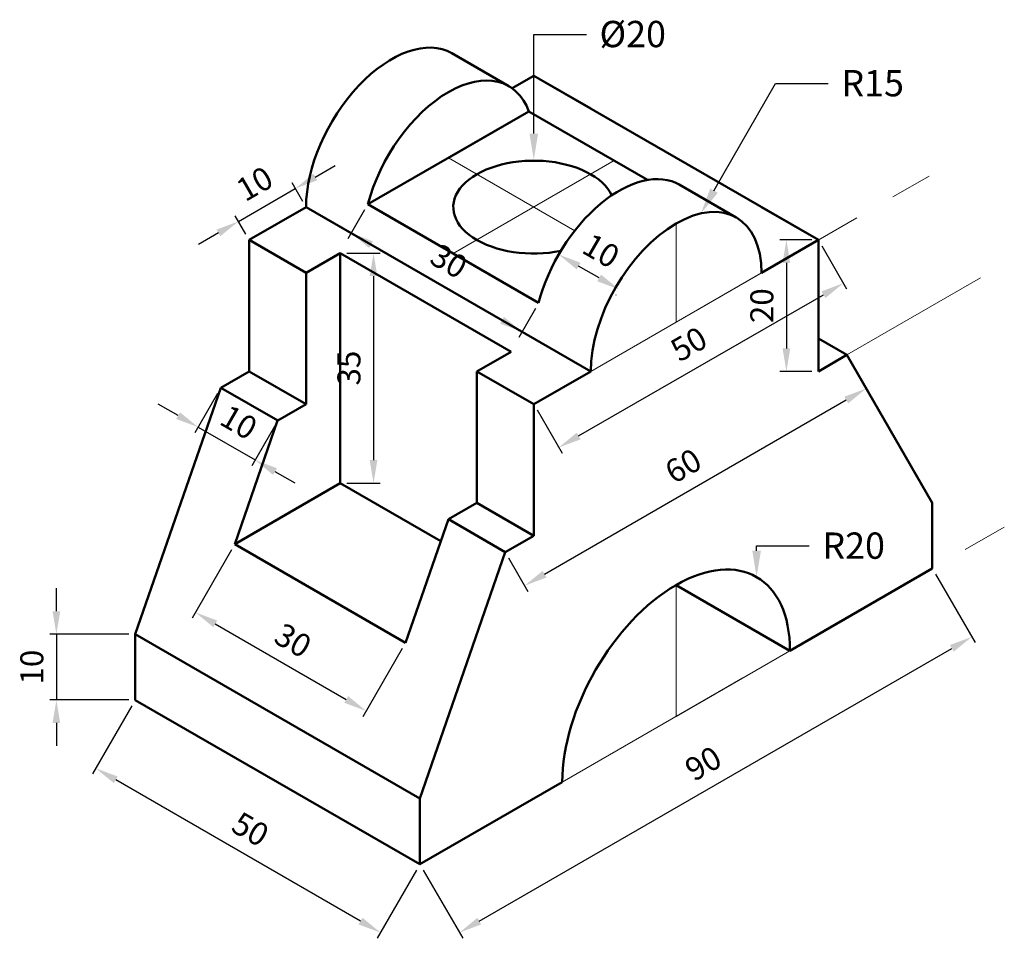
# Model space of a CAD drawing. Units: millimetres. Extents: x 2178 to 2328, y 1178 to 1317.
import ezdxf
from ezdxf import colors
from ezdxf.entities.mleader import LeaderData, LeaderLine
from ezdxf.math import Vec2, Vec3

# ---------------------------------------------------------------- set-up
doc = ezdxf.new("R2010")
doc.units = ezdxf.units.MM
doc.linetypes.add('CENTER', pattern=[50.8, 31.75, -6.35, 6.35, -6.35])
for name, color, linetype, lineweight in [('M-CNTR', 4, 'CENTER', 18), ('M-DIMS', 3, 'Continuous', 25), ('M-OUTL', 7, 'Continuous', 50)]:
    doc.layers.add(name, color=color, linetype=linetype, lineweight=lineweight)
doc.styles.get("Standard").update_dxf_attribs({"font": 'arial.ttf'})
doc.dimstyles.new('AM_ISO$0', dxfattribs={"dimtxt": 3.5, "dimasz": 3.5, "dimexe": 1, "dimexo": 1, "dimgap": 1.5, "dimtad": 1, "dimdsep": 46, "dimtxsty": 'Standard', "dimcen": 0, "dimclrd": 256, "dimclre": 256, "dimclrt": 2, "dimadec": 0, "dimazin": 2, "dimtp": 0.1, "dimtm": 0.1, "dimtfac": 0.71, "dimtdec": 3, "dimtmove": 0, "dimatfit": 3, "dimfxl": 1, "dimlwd": -1, "dimlwe": -1, "dimarcsym": 1})

# ---------------------------------------------------------------- blocks, each defined once
blk = doc.blocks.new('*D3')
at = {"layer": 'Defpoints', "color": 0, "transparency": 16777216}
for p in [(2317.16, 1233.79), (2323.16, 1223.39), (2239.22, 1188.79)]:
    blk.add_point(p, dxfattribs=at)
at = {"layer": 'M-DIMS', "color": 0, "linetype": 'ByBlock', "transparency": 16777216}
for p, q in [((2317.66, 1232.92), (2323.66, 1222.53)), ((2248.25, 1180.14), (2320.13, 1221.64)), ((2239.72, 1187.92), (2245.72, 1177.53))]:
    blk.add_line(p, q, dxfattribs=at)
at = {"layer": 'M-DIMS', "color": 0, "transparency": 16777216}
for points in [[(2319.84, 1222.15), (2320.42, 1221.14), (2323.16, 1223.39)], [(2247.96, 1180.65), (2248.54, 1179.64), (2245.22, 1178.39)]]:
    blk.add_solid(points, dxfattribs=at)
at = {"layer": 'M-DIMS', "color": 0, "transparency": 16777216, "insert": (2282.54, 1203.74), "char_height": 3.5, "attachment_point": 5, "rotation": 30}
blk.add_mtext('90', dxfattribs=at)
blk = doc.blocks.new('*D4')
at = {"layer": 'Defpoints', "color": 0, "transparency": 16777216}
for p in [(2195.91, 1223.79), (2183.91, 1213.79), (2195.91, 1213.79)]:
    blk.add_point(p, dxfattribs=at)
at = {"layer": 'M-DIMS', "color": 0, "linetype": 'ByBlock', "transparency": 16777216}
for p, q in [((2183.91, 1227.29), (2183.91, 1230.79)), ((2194.91, 1223.79), (2182.91, 1223.79)), ((2183.91, 1223.79), (2183.91, 1213.79)), ((2194.91, 1213.79), (2182.91, 1213.79)), ((2183.91, 1210.29), (2183.91, 1206.79))]:
    blk.add_line(p, q, dxfattribs=at)
at = {"layer": 'M-DIMS', "color": 0, "transparency": 16777216}
for points in [[(2183.33, 1227.29), (2184.5, 1227.29), (2183.91, 1223.79)], [(2183.33, 1210.29), (2184.5, 1210.29), (2183.91, 1213.79)]]:
    blk.add_solid(points, dxfattribs=at)
at = {"layer": 'M-DIMS', "color": 0, "transparency": 16777216, "insert": (2180.63, 1218.79), "char_height": 3.5, "attachment_point": 5, "rotation": 90}
blk.add_mtext('10', dxfattribs=at)
blk = doc.blocks.new('*D5')
at = {"layer": 'Defpoints', "color": 0, "transparency": 16777216}
for p in [(2195.91, 1213.79), (2189.91, 1203.39), (2239.22, 1188.79)]:
    blk.add_point(p, dxfattribs=at)
at = {"layer": 'M-DIMS', "color": 0, "linetype": 'ByBlock', "transparency": 16777216}
for p, q in [((2195.41, 1212.92), (2189.41, 1202.53)), ((2230.18, 1180.14), (2192.95, 1201.64)), ((2238.72, 1187.92), (2232.72, 1177.53))]:
    blk.add_line(p, q, dxfattribs=at)
at = {"layer": 'M-DIMS', "color": 0, "transparency": 16777216}
for points in [[(2193.24, 1202.15), (2192.65, 1201.14), (2189.91, 1203.39)], [(2230.48, 1180.65), (2229.89, 1179.64), (2233.22, 1178.39)]]:
    blk.add_solid(points, dxfattribs=at)
at = {"layer": 'M-DIMS', "color": 0, "transparency": 16777216, "insert": (2213.21, 1193.74), "char_height": 3.5, "attachment_point": 5, "rotation": 330}
blk.add_mtext('50', dxfattribs=at)
blk = doc.blocks.new('*D6')
at = {"layer": 'Defpoints', "color": 0, "transparency": 16777216}
for p in [(2227.09, 1281.79), (2227.09, 1246.79), (2232.16, 1246.79)]:
    blk.add_point(p, dxfattribs=at)
at = {"layer": 'M-DIMS', "color": 0, "linetype": 'ByBlock', "transparency": 16777216}
for p, q in [((2228.09, 1281.79), (2233.16, 1281.79)), ((2232.16, 1278.29), (2232.16, 1250.29)), ((2228.09, 1246.79), (2233.16, 1246.79))]:
    blk.add_line(p, q, dxfattribs=at)
at = {"layer": 'M-DIMS', "color": 0, "transparency": 16777216}
for points in [[(2231.57, 1278.29), (2232.74, 1278.29), (2232.16, 1281.79)], [(2231.57, 1250.29), (2232.74, 1250.29), (2232.16, 1246.79)]]:
    blk.add_solid(points, dxfattribs=at)
at = {"layer": 'M-DIMS', "color": 0, "transparency": 16777216, "insert": (2228.87, 1264.29), "char_height": 3.5, "attachment_point": 5, "rotation": 90}
blk.add_mtext('35', dxfattribs=at)
blk = doc.blocks.new('*D7')
at = {"layer": 'Defpoints', "color": 0, "transparency": 16777216}
for p in [(2304.17, 1266.29), (2307.11, 1261.19), (2252.21, 1236.29)]:
    blk.add_point(p, dxfattribs=at)
at = {"layer": 'M-DIMS', "color": 0, "linetype": 'ByBlock', "transparency": 16777216}
for p, q in [((2304.67, 1265.42), (2307.61, 1260.32)), ((2258.18, 1232.94), (2304.08, 1259.44)), ((2252.71, 1235.42), (2255.65, 1230.32))]:
    blk.add_line(p, q, dxfattribs=at)
at = {"layer": 'M-DIMS', "color": 0, "transparency": 16777216}
for points in [[(2303.79, 1259.94), (2304.37, 1258.93), (2307.11, 1261.19)], [(2257.89, 1233.44), (2258.47, 1232.43), (2255.15, 1231.19)]]:
    blk.add_solid(points, dxfattribs=at)
at = {"layer": 'M-DIMS', "color": 0, "transparency": 16777216, "insert": (2279.49, 1249.03), "char_height": 3.5, "attachment_point": 5, "rotation": 30}
blk.add_mtext('60', dxfattribs=at)
blk = doc.blocks.new('*D8')
at = {"layer": 'Defpoints', "color": 0, "transparency": 16777216}
for p in [(2299.84, 1283.79), (2303.63, 1277.21), (2256.54, 1258.79)]:
    blk.add_point(p, dxfattribs=at)
at = {"layer": 'M-DIMS', "color": 0, "linetype": 'ByBlock', "transparency": 16777216}
for p, q in [((2300.34, 1282.92), (2304.13, 1276.34)), ((2263.36, 1253.96), (2300.6, 1275.46)), ((2257.04, 1257.92), (2260.83, 1251.34))]:
    blk.add_line(p, q, dxfattribs=at)
at = {"layer": 'M-DIMS', "color": 0, "transparency": 16777216}
for points in [[(2300.31, 1275.96), (2300.9, 1274.95), (2303.63, 1277.21)], [(2263.07, 1254.46), (2263.66, 1253.45), (2260.33, 1252.21)]]:
    blk.add_solid(points, dxfattribs=at)
at = {"layer": 'M-DIMS', "color": 0, "transparency": 16777216, "insert": (2280.34, 1267.56), "char_height": 3.5, "attachment_point": 5, "rotation": 30}
blk.add_mtext('50', dxfattribs=at)
blk = doc.blocks.new('*D9')
at = {"layer": 'Defpoints', "color": 0, "transparency": 16777216}
for p in [(2208.92, 1261.29), (2217.58, 1256.29), (2214.13, 1250.31)]:
    blk.add_point(p, dxfattribs=at)
at = {"layer": 'M-DIMS', "color": 0, "linetype": 'ByBlock', "transparency": 16777216}
for p, q in [((2208.42, 1260.43), (2204.97, 1254.44)), ((2202.43, 1257.06), (2199.4, 1258.81)), ((2205.47, 1255.31), (2214.13, 1250.31)), ((2217.08, 1255.43), (2213.63, 1249.44)), ((2217.16, 1248.56), (2220.19, 1246.81))]:
    blk.add_line(p, q, dxfattribs=at)
at = {"layer": 'M-DIMS', "color": 0, "transparency": 16777216}
for points in [[(2202.73, 1257.56), (2202.14, 1256.55), (2205.47, 1255.31)], [(2217.45, 1249.06), (2216.87, 1248.05), (2214.13, 1250.31)]]:
    blk.add_solid(points, dxfattribs=at)
at = {"layer": 'M-DIMS', "color": 0, "transparency": 16777216, "insert": (2211.44, 1255.66), "char_height": 3.5, "attachment_point": 5, "rotation": 330}
blk.add_mtext('10', dxfattribs=at)
blk = doc.blocks.new('*D10')
at = {"layer": 'Defpoints', "color": 0, "transparency": 16777216}
for p in [(2220.26, 1291.61), (2221.9, 1288.79), (2213.24, 1283.79)]:
    blk.add_point(p, dxfattribs=at)
at = {"layer": 'M-DIMS', "color": 0, "linetype": 'ByBlock', "transparency": 16777216}
for p, q in [((2223.29, 1293.36), (2226.33, 1295.11)), ((2211.6, 1286.61), (2220.26, 1291.61)), ((2221.4, 1289.65), (2219.76, 1292.48)), ((2212.74, 1284.65), (2211.1, 1287.48)), ((2208.57, 1284.86), (2205.54, 1283.11))]:
    blk.add_line(p, q, dxfattribs=at)
at = {"layer": 'M-DIMS', "color": 0, "transparency": 16777216}
for points in [[(2223, 1293.87), (2223.59, 1292.86), (2220.26, 1291.61)], [(2208.28, 1285.37), (2208.86, 1284.36), (2211.6, 1286.61)]]:
    blk.add_solid(points, dxfattribs=at)
at = {"layer": 'M-DIMS', "color": 0, "transparency": 16777216, "insert": (2214.29, 1291.96), "char_height": 3.5, "attachment_point": 5, "rotation": 30}
blk.add_mtext('10', dxfattribs=at)
blk = doc.blocks.new('*D11')
at = {"layer": 'Defpoints', "color": 0, "transparency": 16777216}
for p in [(2231.3, 1289.21), (2257.28, 1274.21), (2254.74, 1269.82)]:
    blk.add_point(p, dxfattribs=at)
at = {"layer": 'M-DIMS', "color": 0, "linetype": 'ByBlock', "transparency": 16777216}
for p, q in [((2230.8, 1288.35), (2228.26, 1283.95)), ((2231.79, 1283.07), (2251.71, 1271.57)), ((2256.78, 1273.35), (2254.24, 1268.95))]:
    blk.add_line(p, q, dxfattribs=at)
at = {"layer": 'M-DIMS', "color": 0, "transparency": 16777216}
for points in [[(2232.08, 1283.58), (2231.5, 1282.57), (2228.76, 1284.82)], [(2252, 1272.08), (2251.42, 1271.07), (2254.74, 1269.82)]]:
    blk.add_solid(points, dxfattribs=at)
at = {"layer": 'M-DIMS', "color": 0, "transparency": 16777216, "insert": (2243.4, 1280.17), "char_height": 3.5, "attachment_point": 5, "rotation": 330}
blk.add_mtext('30', dxfattribs=at)
blk = doc.blocks.new('*D12')
at = {"layer": 'Defpoints', "color": 0, "transparency": 16777216}
for p in [(2299.84, 1283.79), (2294.97, 1263.79), (2299.84, 1263.79)]:
    blk.add_point(p, dxfattribs=at)
at = {"layer": 'M-DIMS', "color": 0, "linetype": 'ByBlock', "transparency": 16777216}
for p, q in [((2298.84, 1283.79), (2293.97, 1283.79)), ((2294.97, 1280.29), (2294.97, 1267.29)), ((2298.84, 1263.79), (2293.97, 1263.79))]:
    blk.add_line(p, q, dxfattribs=at)
at = {"layer": 'M-DIMS', "color": 0, "transparency": 16777216}
for points in [[(2294.38, 1280.29), (2295.55, 1280.29), (2294.97, 1283.79)], [(2294.38, 1267.29), (2295.55, 1267.29), (2294.97, 1263.79)]]:
    blk.add_solid(points, dxfattribs=at)
at = {"layer": 'M-DIMS', "color": 0, "transparency": 16777216, "insert": (2291.68, 1273.79), "char_height": 3.5, "attachment_point": 5, "rotation": 90}
blk.add_mtext('20', dxfattribs=at)
blk = doc.blocks.new('*D13')
at = {"layer": 'Defpoints', "color": 0, "transparency": 16777216}
for p in [(2211.05, 1237.52), (2237.04, 1222.51), (2231.04, 1212.12)]:
    blk.add_point(p, dxfattribs=at)
at = {"layer": 'M-DIMS', "color": 0, "linetype": 'ByBlock', "transparency": 16777216}
for p, q in [((2210.55, 1236.66), (2204.55, 1226.26)), ((2208.08, 1225.38), (2228.01, 1213.87)), ((2236.54, 1221.65), (2230.54, 1211.25))]:
    blk.add_line(p, q, dxfattribs=at)
at = {"layer": 'M-DIMS', "color": 0, "transparency": 16777216}
for points in [[(2208.37, 1225.88), (2207.79, 1224.87), (2205.05, 1227.13)], [(2228.3, 1214.38), (2227.72, 1213.36), (2231.04, 1212.12)]]:
    blk.add_solid(points, dxfattribs=at)
at = {"layer": 'M-DIMS', "color": 0, "transparency": 16777216, "insert": (2219.69, 1222.47), "char_height": 3.5, "attachment_point": 5, "rotation": 330}
blk.add_mtext('30', dxfattribs=at)
blk = doc.blocks.new('*D14')
at = {"layer": 'Defpoints', "color": 0, "transparency": 16777216}
for p in [(2260.33, 1281.57), (2260.34, 1281.59), (2269.53, 1276.29)]:
    blk.add_point(p, dxfattribs=at)
at = {"layer": 'M-DIMS', "color": 0, "linetype": 'ByBlock', "transparency": 16777216}
for p, q in [((2259.84, 1280.72), (2259.83, 1280.7)), ((2266.48, 1278.01), (2263.36, 1279.82)), ((2269.03, 1275.42), (2269.01, 1275.4))]:
    blk.add_line(p, q, dxfattribs=at)
at = {"layer": 'M-DIMS', "color": 0, "transparency": 16777216}
for points in [[(2263.65, 1280.32), (2263.07, 1279.31), (2260.33, 1281.57)], [(2266.77, 1278.52), (2266.19, 1277.51), (2269.51, 1276.26)]]:
    blk.add_solid(points, dxfattribs=at)
at = {"layer": 'M-DIMS', "color": 0, "transparency": 16777216, "insert": (2266.56, 1281.76), "char_height": 3.5, "attachment_point": 5, "rotation": 330}
blk.add_mtext('10', dxfattribs=at)

msp = doc.modelspace()

# ---------------------------------------------------------------- linework, layer by layer
at = {"layer": 'M-CNTR'}
for p, q in [((2243.546, 1296.285), (2262.765, 1285.189)), ((2244.289, 1281.714), (2268.784, 1295.856)), ((2278.187, 1271.285), (2317.66, 1294.075)), ((2278.187, 1271.285), (2278.187, 1286.285)), ((2265.197, 1263.785), (2291.177, 1278.785)), ((2304.168, 1266.285), (2324.476, 1278.01)), ((2278.187, 1211.285), (2328.115, 1240.111)), ((2278.187, 1211.285), (2278.187, 1231.285)), ((2260.866, 1201.285), (2295.507, 1221.285))]:
    msp.add_line(p, q, dxfattribs=at)
at = {"layer": 'M-OUTL'}
for p, q in [((2244.071, 1312.195), (2252.732, 1307.195)), ((2253.228, 1306.875), (2256.536, 1308.785)), ((2256.536, 1308.785), (2265.197, 1303.785)), ((2299.838, 1283.785), (2256.536, 1308.785)), ((2255.793, 1303.356), (2231.299, 1289.214)), ((2243.546, 1296.285), (2255.793, 1303.356)), ((2255.793, 1303.356), (2273.857, 1292.927)), ((2287.327, 1287.221), (2278.667, 1292.221)), ((2221.895, 1288.785), (2213.235, 1283.785)), ((2213.235, 1283.785), (2221.895, 1288.785)), ((2221.895, 1288.785), (2265.197, 1263.785)), ((2221.895, 1288.785), (2230.556, 1283.785)), ((2231.299, 1289.214), (2257.279, 1274.214)), ((2299.838, 1283.785), (2291.177, 1288.785)), ((2287.327, 1287.221), (2287.373, 1287.195)), ((2213.235, 1283.785), (2213.235, 1263.785)), ((2213.235, 1283.785), (2221.895, 1278.785)), ((2291.177, 1278.785), (2299.838, 1283.785)), ((2299.838, 1283.785), (2291.177, 1278.785)), ((2299.838, 1283.785), (2299.838, 1263.785)), ((2221.895, 1278.785), (2227.091, 1281.785)), ((2227.091, 1281.785), (2253.072, 1266.785)), ((2227.091, 1281.785), (2227.091, 1246.785)), ((2221.895, 1278.785), (2221.895, 1258.785)), ((2304.168, 1266.285), (2299.838, 1268.785)), ((2253.072, 1266.785), (2247.876, 1263.785)), ((2299.838, 1263.785), (2304.168, 1266.285)), ((2317.158, 1243.785), (2304.168, 1266.285)), ((2213.235, 1263.785), (2208.905, 1261.285)), ((2208.921, 1261.294), (2213.235, 1263.785)), ((2221.911, 1258.794), (2213.235, 1263.785)), ((2247.876, 1263.785), (2247.86, 1243.776)), ((2247.876, 1263.785), (2256.536, 1258.785)), ((2265.197, 1263.785), (2256.536, 1258.785)), ((2208.905, 1261.285), (2195.915, 1223.785)), ((2217.581, 1256.294), (2208.921, 1261.294)), ((2221.911, 1258.794), (2217.581, 1256.294)), ((2256.536, 1258.785), (2256.536, 1238.785)), ((2217.549, 1256.294), (2211.046, 1237.521)), ((2227.091, 1246.785), (2211.046, 1237.521)), ((2227.091, 1246.785), (2242.391, 1237.952)), ((2243.546, 1241.285), (2247.86, 1243.776)), ((2256.536, 1238.785), (2247.86, 1243.776)), ((2317.158, 1233.785), (2317.158, 1243.785)), ((2243.546, 1241.285), (2237.043, 1222.512)), ((2252.206, 1236.285), (2243.546, 1241.285)), ((2256.536, 1238.785), (2252.206, 1236.285)), ((2211.046, 1237.521), (2237.043, 1222.512)), ((2252.206, 1236.285), (2239.216, 1198.785)), ((2295.507, 1221.285), (2317.158, 1233.785)), ((2295.508, 1221.285), (2278.187, 1231.285)), ((2195.915, 1213.785), (2195.915, 1223.785)), ((2195.915, 1223.785), (2239.216, 1198.785)), ((2195.915, 1213.785), (2239.216, 1188.785)), ((2239.216, 1188.785), (2260.866, 1201.285)), ((2239.216, 1198.785), (2239.216, 1188.785))]:
    msp.add_line(p, q, dxfattribs=at)
for centre, major_axis, start_param, end_param in [((2234.886, 1296.285), (-9.186, -15.91), 3.1415927, 5.4977871), ((2243.546, 1291.285), (-9.186, -15.91), 2.6960314, 5.1579502), ((2256.536, 1288.785), (-12.247, 0), 3.3967046, 8.1973003), ((2269.527, 1276.285), (-9.186, -15.91), 3.136626, 5.1579502), ((2278.187, 1271.285), (-9.186, -15.91), 2.3561945, 5.4977871), ((2278.187, 1211.285), (-12.247, -21.213), 2.3561945, 5.4977871)]:
    msp.add_ellipse(centre, major_axis=major_axis, ratio=0.5773503, start_param=start_param, end_param=end_param, dxfattribs=at)

# ---------------------------------------------------------------- dimensions: what is measured, and where the dimension line sits
at = {"layer": 'M-DIMS'}
for p1, p2, distance, override, picture, middle in [((2213.235, 1283.785), (2221.895, 1288.785), 3.265, {"dimclrd": 0, "dimclre": 0, "dimclrt": 0}, '*D10', (2214.289, 1291.959)), ((2231.299, 1289.214), (2257.279, 1274.214), -5.073, {"dimpost": '', "dimclrd": 0, "dimclre": 0, "dimclrt": 0}, '*D11', (2243.396, 1280.168)), ((2256.536, 1258.785), (2299.838, 1283.785), -7.594, {"dimclrd": 0, "dimclre": 0, "dimclrt": 0}, '*D8', (2280.34, 1267.555)), ((2299.838, 1283.785), (2299.838, 1263.785), -4.869, {"dimclrd": 0, "dimclre": 0, "dimclrt": 0}, '*D12', (2291.681, 1273.785)), ((2227.091, 1281.785), (2227.091, 1246.785), 5.064, {"dimpost": '', "dimclrd": 0, "dimclre": 0, "dimclrt": 0}, '*D6', (2228.867, 1264.285)), ((2252.206, 1236.285), (2304.168, 1266.285), -5.887, {"dimclrd": 0, "dimclre": 0, "dimclrt": 0}, '*D7', (2279.487, 1249.034)), ((2208.921, 1261.294), (2217.581, 1256.294), -6.911, {"dimpost": '', "dimclrd": 0, "dimclre": 0, "dimclrt": 0}, '*D9', (2211.439, 1255.656)), ((2239.216, 1188.785), (2317.158, 1233.785), -12, {"dimpost": '', "dimclrd": 0, "dimclre": 0, "dimclrt": 0}, '*D3', (2282.543, 1203.74)), ((2195.915, 1223.785), (2195.915, 1213.785), -12, {"dimclrd": 0, "dimclre": 0, "dimclrt": 0}, '*D4', (2180.628, 1218.785)), ((2239.216, 1188.785), (2195.915, 1213.785), 12, {"dimclrd": 0, "dimclre": 0, "dimclrt": 0}, '*D5', (2213.209, 1193.74))]:
    dim = msp.add_aligned_dim(p1=p1, p2=p2, distance=distance, dimstyle='AM_ISO$0', override=override, dxfattribs=at)
    dim.commit()
    dim.dimension.update_dxf_attribs({"geometry": picture, "text_midpoint": middle})
for p1, p2, distance, text, picture, middle in [((2269.527, 1276.285), (2260.341, 1281.589), 0.026, '10', '*D14', (2266.565, 1281.761)), ((2211.046, 1237.521), (2237.043, 1222.512), -12, '30', '*D13', (2219.688, 1222.472))]:
    dim = msp.add_aligned_dim(p1=p1, p2=p2, distance=distance, text=text, dimstyle='AM_ISO$0', override={"dimpost": '', "dimclrd": 0, "dimclre": 0, "dimclrt": 0}, dxfattribs=at)
    dim.commit()
    dim.dimension.update_dxf_attribs({"geometry": picture, "text_midpoint": middle})

# ---------------------------------------------------------------- leaders
ml = msp.add_multileader_mtext('Standard', dxfattribs=at)
ml.set_content('{\\C2;%%C20}', color=256)
ml.set_leader_properties()
ml.build(insert=Vec2(0, 0))
ctx = ml.context
ctx.base_point, ctx.plane_origin = Vec3(2264.536, 1315.04), Vec3(2256.536, 1295.977)
notes = []
notes.append((ctx, [(0, (1, 1, 0), (2256.536, 1315.04), (1, 0), 8, [(0, [(2256.536, 1295.977)], 0, [])])]))
ctx.mtext.insert, ctx.mtext.flow_direction = Vec3(2266.536, 1317.121), 5
ml = msp.add_multileader_mtext('Standard', dxfattribs=at)
ml.set_content('{\\C2;R15}', color=256)
ml.set_leader_properties()
ml.build(insert=Vec2(0, 0))
ctx = ml.context
ctx.base_point, ctx.plane_origin = Vec3(2301.325, 1307.611), Vec3(2281.958, 1287.816)
notes.append((ctx, [(0, (1, 1, 0), (2293.325, 1307.611), (1, 0), 8, [(0, [(2281.958, 1287.816)], 0, [])])]))
ctx.mtext.insert, ctx.mtext.flow_direction = Vec3(2303.325, 1309.645), 5
ml = msp.add_multileader_mtext('Standard', dxfattribs=at)
ml.set_content('{\\C2;R20}', color=256)
ml.set_leader_properties()
ml.build(insert=Vec2(0, 0))
ctx = ml.context
ctx.base_point, ctx.plane_origin = Vec3(2298.434, 1237.243), Vec3(2290.434, 1232.498)
notes.append((ctx, [(0, (1, 1, 0), (2290.434, 1237.243), (1, 0), 8, [(0, [(2290.434, 1232.498)], 0, [])])]))
ctx.mtext.insert, ctx.mtext.flow_direction = Vec3(2300.434, 1239.277), 5
for ctx, leaders in notes:
    for number, flags, end, landing, length, lines in leaders:
        leader = LeaderData()
        leader.index, (leader.has_last_leader_line, leader.has_dogleg_vector, leader.attachment_direction) = number, flags
        leader.last_leader_point, leader.dogleg_vector, leader.dogleg_length = Vec3(end), Vec3(landing), length
        for number, points, colour, breaks in lines:
            line = LeaderLine()
            line.index, line.vertices, line.color, line.breaks = number, Vec3.list(points), colors.encode_raw_color(colour), breaks
            leader.lines.append(line)
        ctx.leaders.append(leader)

doc.saveas('drawing.dxf')
